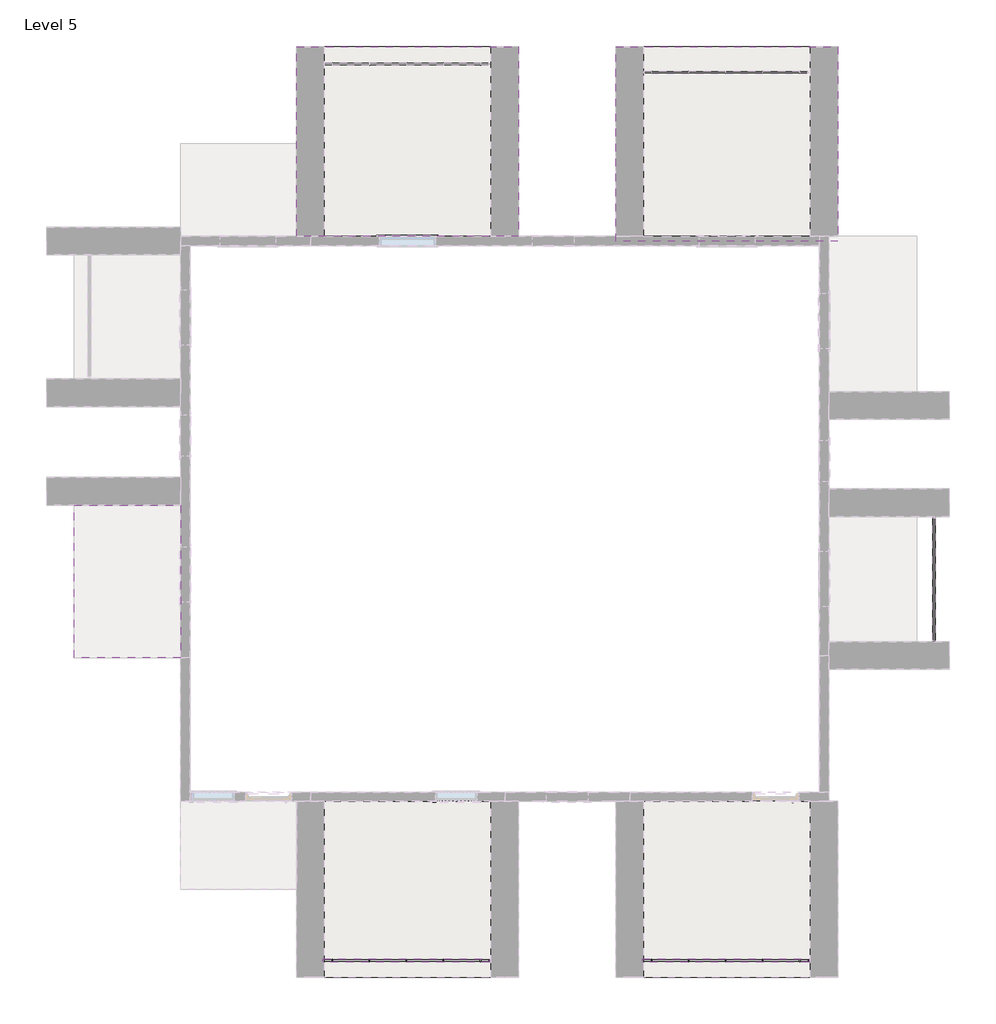
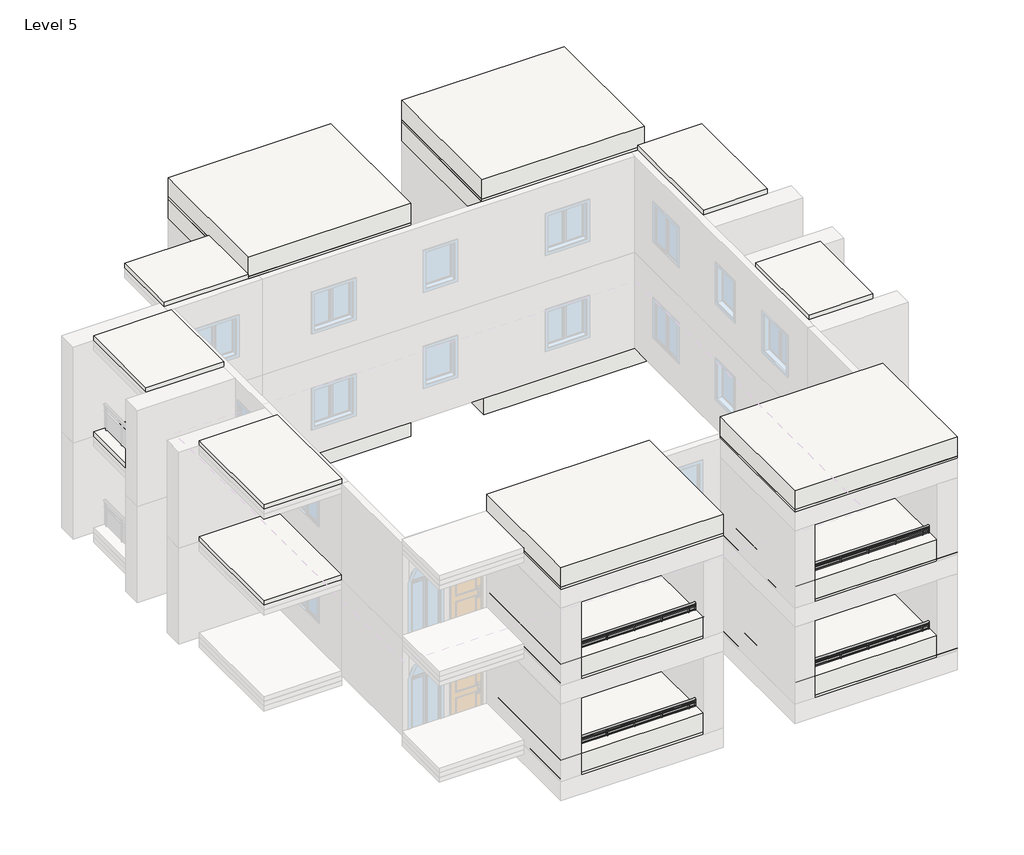
# One storey, part 3 of 4: 14 slabs, 5 railings.
"""IFC4 building model written with IfcOpenShell, lengths in millimetres."""

from ifc_helpers import new_model, si_unit, point, frame, origin, place, context, project, spatial, polyline, ellipse_curve, trimmed, outline, extrude, element, save
from ifc_brep_helpers import plane_surface, extruded_surface, advanced_brep

model = new_model("IFC4")

# Units and contexts
model_context = context("Model", 3, world=origin())
ifc_project = project(units=[si_unit("LENGTHUNIT", "METRE", prefix="MILLI")], contexts=[model_context])

# Site, building, storey
site = spatial("IfcSite", under=ifc_project)
building = spatial("IfcBuilding", under=site)
storey = spatial("IfcBuildingStorey", under=building, Name="Level 5", Elevation=12192.0)

# Railings
placement = place(None, origin())
element("IfcRailing", 1, ObjectType="Glass Panel - Bottom Fill", at=placement, inside=storey, context=model_context, shape_type="SolidModel", body=[
    advanced_brep(
    [(-9258.4937431, -9324.2034265, 13411.2), (-9258.4937431, -9400.4034265, 13411.2), (-5600.8937431, -9324.2034265, 13411.2), (-5600.8937431, -9400.4034265, 13411.2)],
    [
        (0, 1, ellipse_curve(frame((-9258.4937431, -9362.3034265, 13411.2), z_axis=(-1.0, 0.0, 0.0), x_axis=(0.0, -1.0, 0.0)), 38.1, 28.575)),
        (1, 0, ellipse_curve(frame((-9258.4937431, -9362.3034265, 13411.2), z_axis=(-1.0, 0.0, 0.0), x_axis=(0.0, -1.0, 0.0)), 38.1, 28.575)),
        (2, 3, ellipse_curve(frame((-5600.8937431, -9362.3034265, 13411.2), z_axis=(1.0, 0.0, 0.0), x_axis=(0.0, -1.0, 0.0)), 38.1, 28.575)),
        (3, 2, ellipse_curve(frame((-5600.8937431, -9362.3034265, 13411.2), z_axis=(1.0, 0.0, 0.0), x_axis=(0.0, -1.0, 0.0)), 38.1, 28.575)),
        (0, 2),
        (3, 1),
    ],
    [
        plane_surface(frame((-9258.4937431, -9362.3034265, 13411.2), z_axis=(-1.0, 0.0, 0.0), x_axis=(0.0, 1.0, 0.0))),
        plane_surface(frame((-5600.8937431, -9362.3034265, 13411.2), z_axis=(1.0, 0.0, 0.0), x_axis=(0.0, 1.0, 0.0))),
        extruded_surface(trimmed(ellipse_curve(frame((-5600.8937431, -9362.3034265, 13411.2), z_axis=(-1.0, 0.0, 0.0), x_axis=(0.0, -1.0, 0.0)), 38.1, 28.575), [point((-5600.8937431, -9324.2034265, 13411.2))], [point((-5600.8937431, -9400.4034265, 13411.2))], True, "CARTESIAN"), (-3657.5999999999995, 0.0, 0.0), 3657.5999999999995),
        extruded_surface(trimmed(ellipse_curve(frame((-5600.8937431, -9362.3034265, 13411.2), z_axis=(-1.0, 0.0, 0.0), x_axis=(0.0, -1.0, 0.0)), 38.1, 28.575), [point((-5600.8937431, -9400.4034265, 13411.2))], [point((-5600.8937431, -9324.2034265, 13411.2))], True, "CARTESIAN"), (-3657.5999999999995, 0.0, 0.0), 3657.5999999999995),
    ],
    [
        (0, [[1, 2]]),
        (1, [[3, 4]]),
        (2, [[-1, 5, -4, 6]]),
        (3, [[-2, -6, -3, -5]]),
    ],
),
    extrude(outline(polyline([(-9258.4937431, -9375.0034265), (-9258.4937431, -9349.6034265), (-5600.8937431, -9349.6034265), (-5600.8937431, -9375.0034265), (-9258.4937431, -9375.0034265)])), frame((0.0, 0.0, 13296.9), z_axis=(0.0, 0.0, 1.0), x_axis=(1.0, 0.0, 0.0)), (0.0, 0.0, 1.0), 25.4),
    extrude(outline(polyline([(-9258.4937431, -9375.0034265), (-9258.4937431, -9349.6034265), (-5600.8937431, -9349.6034265), (-5600.8937431, -9375.0034265), (-9258.4937431, -9375.0034265)])), frame((0.0, 0.0, 13195.3), z_axis=(0.0, 0.0, 1.0), x_axis=(1.0, 0.0, 0.0)), (0.0, 0.0, 1.0), 25.4),
    extrude(outline(polyline([(-5810.4437431, -9387.7034265), (-5810.4437431, -9336.9034265), (-5797.7437431, -9336.9034265), (-5797.7437431, -9387.7034265), (-5810.4437431, -9387.7034265)])), frame((0.0, 0.0, 12496.8), z_axis=(0.0, 0.0, 1.0), x_axis=(1.0, 0.0, 0.0)), (0.0, 0.0, 1.0), 885.6788223),
    extrude(outline(polyline([(-6616.8937431, -9355.7682695), (-5804.0937431, -9355.7682695), (-5804.0937431, -9362.1182695), (-6616.8937431, -9362.1182695), (-6616.8937431, -9355.7682695)])), frame((0.0, 0.0, 12598.4), z_axis=(0.0, 0.0, 1.0), x_axis=(1.0, 0.0, 0.0)), (0.0, 0.0, 1.0), 596.9),
    extrude(outline(polyline([(-6623.2437431, -9387.7034265), (-6623.2437431, -9336.9034265), (-6610.5437431, -9336.9034265), (-6610.5437431, -9387.7034265), (-6623.2437431, -9387.7034265)])), frame((0.0, 0.0, 12496.8), z_axis=(0.0, 0.0, 1.0), x_axis=(1.0, 0.0, 0.0)), (0.0, 0.0, 1.0), 885.6788223),
    extrude(outline(polyline([(-7429.6937431, -9355.7682695), (-6616.8937431, -9355.7682695), (-6616.8937431, -9362.1182695), (-7429.6937431, -9362.1182695), (-7429.6937431, -9355.7682695)])), frame((0.0, 0.0, 12598.4), z_axis=(0.0, 0.0, 1.0), x_axis=(1.0, 0.0, 0.0)), (0.0, 0.0, 1.0), 596.9),
    extrude(outline(polyline([(-7436.0437431, -9387.7034265), (-7436.0437431, -9336.9034265), (-7423.3437431, -9336.9034265), (-7423.3437431, -9387.7034265), (-7436.0437431, -9387.7034265)])), frame((0.0, 0.0, 12496.8), z_axis=(0.0, 0.0, 1.0), x_axis=(1.0, 0.0, 0.0)), (0.0, 0.0, 1.0), 885.6788223),
    extrude(outline(polyline([(-8242.4937431, -9355.7682695), (-7429.6937431, -9355.7682695), (-7429.6937431, -9362.1182695), (-8242.4937431, -9362.1182695), (-8242.4937431, -9355.7682695)])), frame((0.0, 0.0, 12598.4), z_axis=(0.0, 0.0, 1.0), x_axis=(1.0, 0.0, 0.0)), (0.0, 0.0, 1.0), 596.9),
    extrude(outline(polyline([(-8248.8437431, -9387.7034265), (-8248.8437431, -9336.9034265), (-8236.1437431, -9336.9034265), (-8236.1437431, -9387.7034265), (-8248.8437431, -9387.7034265)])), frame((0.0, 0.0, 12496.8), z_axis=(0.0, 0.0, 1.0), x_axis=(1.0, 0.0, 0.0)), (0.0, 0.0, 1.0), 885.6788223),
    extrude(outline(polyline([(-9055.2937431, -9355.7682695), (-8242.4937431, -9355.7682695), (-8242.4937431, -9362.1182695), (-9055.2937431, -9362.1182695), (-9055.2937431, -9355.7682695)])), frame((0.0, 0.0, 12598.4), z_axis=(0.0, 0.0, 1.0), x_axis=(1.0, 0.0, 0.0)), (0.0, 0.0, 1.0), 596.9),
    extrude(outline(polyline([(-9061.6437431, -9387.7034265), (-9061.6437431, -9336.9034265), (-9048.9437431, -9336.9034265), (-9048.9437431, -9387.7034265), (-9061.6437431, -9387.7034265)])), frame((0.0, 0.0, 12496.8), z_axis=(0.0, 0.0, 1.0), x_axis=(1.0, 0.0, 0.0)), (0.0, 0.0, 1.0), 885.6788223),
    extrude(outline(polyline([(-5613.5937431, -9371.8284265), (-5613.5937431, -9352.7784265), (-5594.5437431, -9352.7784265), (-5594.5437431, -9371.8284265), (-5613.5937431, -9371.8284265)])), frame((0.0, 0.0, 12496.8), z_axis=(0.0, 0.0, 1.0), x_axis=(1.0, 0.0, 0.0)), (0.0, 0.0, 1.0), 885.6788223),
    extrude(outline(polyline([(-9264.8437431, -9371.8284265), (-9264.8437431, -9352.7784265), (-9245.7937431, -9352.7784265), (-9245.7937431, -9371.8284265), (-9264.8437431, -9371.8284265)])), frame((0.0, 0.0, 12496.8), z_axis=(0.0, 0.0, 1.0), x_axis=(1.0, 0.0, 0.0)), (0.0, 0.0, 1.0), 885.6788223),
])
element("IfcRailing", 2, ObjectType="Glass Panel - Bottom Fill", at=placement, inside=storey, context=model_context, shape_type="SolidModel", body=[
    advanced_brep(
    [(-2248.0325613, -9324.2034265, 13406.1393423), (-2248.0325613, -9400.4034265, 13406.1393423), (1409.5674387, -9324.2034265, 13406.1393423), (1409.5674387, -9400.4034265, 13406.1393423)],
    [
        (0, 1, ellipse_curve(frame((-2248.0325613, -9362.3034265, 13406.1393423), z_axis=(-1.0, 0.0, 0.0), x_axis=(0.0, -1.0, 0.0)), 38.1, 28.575)),
        (1, 0, ellipse_curve(frame((-2248.0325613, -9362.3034265, 13406.1393423), z_axis=(-1.0, 0.0, 0.0), x_axis=(0.0, -1.0, 0.0)), 38.1, 28.575)),
        (2, 3, ellipse_curve(frame((1409.5674387, -9362.3034265, 13406.1393423), z_axis=(1.0, 0.0, 0.0), x_axis=(0.0, -1.0, 0.0)), 38.1, 28.575)),
        (3, 2, ellipse_curve(frame((1409.5674387, -9362.3034265, 13406.1393423), z_axis=(1.0, 0.0, 0.0), x_axis=(0.0, -1.0, 0.0)), 38.1, 28.575)),
        (0, 2),
        (3, 1),
    ],
    [
        plane_surface(frame((-2248.0325613, -9362.3034265, 13406.1393423), z_axis=(-1.0, 0.0, 0.0), x_axis=(0.0, 1.0, 0.0))),
        plane_surface(frame((1409.5674387, -9362.3034265, 13406.1393423), z_axis=(1.0, 0.0, 0.0), x_axis=(0.0, 1.0, 0.0))),
        extruded_surface(trimmed(ellipse_curve(frame((1409.5674387, -9362.3034265, 13406.1393423), z_axis=(-1.0, 0.0, 0.0), x_axis=(0.0, -1.0, 0.0)), 38.1, 28.575), [point((1409.5674387, -9324.2034265, 13406.1393423))], [point((1409.5674387, -9400.4034265, 13406.1393423))], True, "CARTESIAN"), (-3657.6, 0.0, 0.0), 3657.6),
        extruded_surface(trimmed(ellipse_curve(frame((1409.5674387, -9362.3034265, 13406.1393423), z_axis=(-1.0, 0.0, 0.0), x_axis=(0.0, -1.0, 0.0)), 38.1, 28.575), [point((1409.5674387, -9400.4034265, 13406.1393423))], [point((1409.5674387, -9324.2034265, 13406.1393423))], True, "CARTESIAN"), (-3657.6, 0.0, 0.0), 3657.6),
    ],
    [
        (0, [[1, 2]]),
        (1, [[3, 4]]),
        (2, [[-1, 5, -4, 6]]),
        (3, [[-2, -6, -3, -5]]),
    ],
),
    extrude(outline(polyline([(-2248.0325613, -9375.0034265), (-2248.0325613, -9349.6034265), (1409.5674387, -9349.6034265), (1409.5674387, -9375.0034265), (-2248.0325613, -9375.0034265)])), frame((0.0, 0.0, 13291.8393423), z_axis=(0.0, 0.0, 1.0), x_axis=(1.0, 0.0, 0.0)), (0.0, 0.0, 1.0), 25.4),
    extrude(outline(polyline([(-2248.0325613, -9375.0034265), (-2248.0325613, -9349.6034265), (1409.5674387, -9349.6034265), (1409.5674387, -9375.0034265), (-2248.0325613, -9375.0034265)])), frame((0.0, 0.0, 13190.2393423), z_axis=(0.0, 0.0, 1.0), x_axis=(1.0, 0.0, 0.0)), (0.0, 0.0, 1.0), 25.4),
    extrude(outline(polyline([(1200.0174387, -9387.7034265), (1200.0174387, -9336.9034265), (1212.7174387, -9336.9034265), (1212.7174387, -9387.7034265), (1200.0174387, -9387.7034265)])), frame((0.0, 0.0, 12491.7393423), z_axis=(0.0, 0.0, 1.0), x_axis=(1.0, 0.0, 0.0)), (0.0, 0.0, 1.0), 885.6788223),
    extrude(outline(polyline([(393.5674387, -9355.7682695), (1206.3674387, -9355.7682695), (1206.3674387, -9362.1182695), (393.5674387, -9362.1182695), (393.5674387, -9355.7682695)])), frame((0.0, 0.0, 12593.3393423), z_axis=(0.0, 0.0, 1.0), x_axis=(1.0, 0.0, 0.0)), (0.0, 0.0, 1.0), 596.9),
    extrude(outline(polyline([(387.2174387, -9387.7034265), (387.2174387, -9336.9034265), (399.9174387, -9336.9034265), (399.9174387, -9387.7034265), (387.2174387, -9387.7034265)])), frame((0.0, 0.0, 12491.7393423), z_axis=(0.0, 0.0, 1.0), x_axis=(1.0, 0.0, 0.0)), (0.0, 0.0, 1.0), 885.6788223),
    extrude(outline(polyline([(-419.2325613, -9355.7682695), (393.5674387, -9355.7682695), (393.5674387, -9362.1182695), (-419.2325613, -9362.1182695), (-419.2325613, -9355.7682695)])), frame((0.0, 0.0, 12593.3393423), z_axis=(0.0, 0.0, 1.0), x_axis=(1.0, 0.0, 0.0)), (0.0, 0.0, 1.0), 596.9),
    extrude(outline(polyline([(-425.5825613, -9387.7034265), (-425.5825613, -9336.9034265), (-412.8825613, -9336.9034265), (-412.8825613, -9387.7034265), (-425.5825613, -9387.7034265)])), frame((0.0, 0.0, 12491.7393423), z_axis=(0.0, 0.0, 1.0), x_axis=(1.0, 0.0, 0.0)), (0.0, 0.0, 1.0), 885.6788223),
    extrude(outline(polyline([(-1232.0325613, -9355.7682695), (-419.2325613, -9355.7682695), (-419.2325613, -9362.1182695), (-1232.0325613, -9362.1182695), (-1232.0325613, -9355.7682695)])), frame((0.0, 0.0, 12593.3393423), z_axis=(0.0, 0.0, 1.0), x_axis=(1.0, 0.0, 0.0)), (0.0, 0.0, 1.0), 596.9),
    extrude(outline(polyline([(-1238.3825613, -9387.7034265), (-1238.3825613, -9336.9034265), (-1225.6825613, -9336.9034265), (-1225.6825613, -9387.7034265), (-1238.3825613, -9387.7034265)])), frame((0.0, 0.0, 12491.7393423), z_axis=(0.0, 0.0, 1.0), x_axis=(1.0, 0.0, 0.0)), (0.0, 0.0, 1.0), 885.6788223),
    extrude(outline(polyline([(-2044.8325613, -9355.7682695), (-1232.0325613, -9355.7682695), (-1232.0325613, -9362.1182695), (-2044.8325613, -9362.1182695), (-2044.8325613, -9355.7682695)])), frame((0.0, 0.0, 12593.3393423), z_axis=(0.0, 0.0, 1.0), x_axis=(1.0, 0.0, 0.0)), (0.0, 0.0, 1.0), 596.9),
    extrude(outline(polyline([(-2051.1825613, -9387.7034265), (-2051.1825613, -9336.9034265), (-2038.4825613, -9336.9034265), (-2038.4825613, -9387.7034265), (-2051.1825613, -9387.7034265)])), frame((0.0, 0.0, 12491.7393423), z_axis=(0.0, 0.0, 1.0), x_axis=(1.0, 0.0, 0.0)), (0.0, 0.0, 1.0), 885.6788223),
    extrude(outline(polyline([(1396.8674387, -9371.8284265), (1396.8674387, -9352.7784265), (1415.9174387, -9352.7784265), (1415.9174387, -9371.8284265), (1396.8674387, -9371.8284265)])), frame((0.0, 0.0, 12491.7393423), z_axis=(0.0, 0.0, 1.0), x_axis=(1.0, 0.0, 0.0)), (0.0, 0.0, 1.0), 885.6788223),
    extrude(outline(polyline([(-2254.3825613, -9371.8284265), (-2254.3825613, -9352.7784265), (-2235.3325613, -9352.7784265), (-2235.3325613, -9371.8284265), (-2254.3825613, -9371.8284265)])), frame((0.0, 0.0, 12491.7393423), z_axis=(0.0, 0.0, 1.0), x_axis=(1.0, 0.0, 0.0)), (0.0, 0.0, 1.0), 885.6788223),
])
element("IfcRailing", 3, ObjectType="Glass Panel - Bottom Fill", at=placement, inside=storey, context=model_context, shape_type="SolidModel", body=[
    advanced_brep(
    [(4190.8062569, 350.013611, 13411.2), (4114.6062569, 350.013611, 13411.2), (4190.8062569, -2342.386389, 13411.2), (4114.6062569, -2342.386389, 13411.2)],
    [
        (0, 1, ellipse_curve(frame((4152.7062569, 350.013611, 13411.2), z_axis=(0.0, 1.0, 0.0), x_axis=(-1.0, 0.0, 0.0)), 38.1, 28.575)),
        (1, 0, ellipse_curve(frame((4152.7062569, 350.013611, 13411.2), z_axis=(0.0, 1.0, 0.0), x_axis=(-1.0, 0.0, 0.0)), 38.1, 28.575)),
        (2, 3, ellipse_curve(frame((4152.7062569, -2342.386389, 13411.2), z_axis=(0.0, -1.0, 0.0), x_axis=(-1.0, 0.0, 0.0)), 38.1, 28.575)),
        (3, 2, ellipse_curve(frame((4152.7062569, -2342.386389, 13411.2), z_axis=(0.0, -1.0, 0.0), x_axis=(-1.0, 0.0, 0.0)), 38.1, 28.575)),
        (0, 2),
        (3, 1),
    ],
    [
        plane_surface(frame((4152.7062569, 350.013611, 13411.2), z_axis=(0.0, 1.0, 0.0), x_axis=(0.0, 0.0, -1.0))),
        plane_surface(frame((4152.7062569, -2342.386389, 13411.2), z_axis=(0.0, -1.0, 0.0), x_axis=(0.0, 0.0, -1.0))),
        extruded_surface(trimmed(ellipse_curve(frame((4152.7062569, -2342.386389, 13411.2), z_axis=(0.0, 1.0, 0.0), x_axis=(-1.0, 0.0, 0.0)), 38.1, 28.575), [point((4190.8062569, -2342.386389, 13411.2))], [point((4114.6062569, -2342.386389, 13411.2))], True, "CARTESIAN"), (0.0, 2692.3999999999996, 0.0), 2692.3999999999996),
        extruded_surface(trimmed(ellipse_curve(frame((4152.7062569, -2342.386389, 13411.2), z_axis=(0.0, 1.0, 0.0), x_axis=(-1.0, 0.0, 0.0)), 38.1, 28.575), [point((4114.6062569, -2342.386389, 13411.2))], [point((4190.8062569, -2342.386389, 13411.2))], True, "CARTESIAN"), (0.0, 2692.3999999999996, 0.0), 2692.3999999999996),
    ],
    [
        (0, [[1, 2]]),
        (1, [[3, 4]]),
        (2, [[-1, 5, -4, 6]]),
        (3, [[-2, -6, -3, -5]]),
    ],
),
    extrude(outline(polyline([(4140.0062569, 350.013611), (4165.4062569, 350.013611), (4165.4062569, -2342.386389), (4140.0062569, -2342.386389), (4140.0062569, 350.013611)])), frame((0.0, 0.0, 13296.9), z_axis=(0.0, 0.0, 1.0), x_axis=(1.0, 0.0, 0.0)), (0.0, 0.0, 1.0), 25.4),
    extrude(outline(polyline([(4140.0062569, 350.013611), (4165.4062569, 350.013611), (4165.4062569, -2342.386389), (4140.0062569, -2342.386389), (4140.0062569, 350.013611)])), frame((0.0, 0.0, 13195.3), z_axis=(0.0, 0.0, 1.0), x_axis=(1.0, 0.0, 0.0)), (0.0, 0.0, 1.0), 25.4),
    extrude(outline(polyline([(4127.3062569, -2209.036389), (4178.1062569, -2209.036389), (4178.1062569, -2221.736389), (4127.3062569, -2221.736389), (4127.3062569, -2209.036389)])), frame((0.0, 0.0, 12496.8), z_axis=(0.0, 0.0, 1.0), x_axis=(1.0, 0.0, 0.0)), (0.0, 0.0, 1.0), 885.6788223),
    extrude(outline(polyline([(4159.2414139, -1402.586389), (4159.2414139, -2215.386389), (4152.8914139, -2215.386389), (4152.8914139, -1402.586389), (4159.2414139, -1402.586389)])), frame((0.0, 0.0, 12598.4), z_axis=(0.0, 0.0, 1.0), x_axis=(1.0, 0.0, 0.0)), (0.0, 0.0, 1.0), 596.9),
    extrude(outline(polyline([(4127.3062569, -1396.236389), (4178.1062569, -1396.236389), (4178.1062569, -1408.936389), (4127.3062569, -1408.936389), (4127.3062569, -1396.236389)])), frame((0.0, 0.0, 12496.8), z_axis=(0.0, 0.0, 1.0), x_axis=(1.0, 0.0, 0.0)), (0.0, 0.0, 1.0), 885.6788223),
    extrude(outline(polyline([(4159.2414139, -589.786389), (4159.2414139, -1402.586389), (4152.8914139, -1402.586389), (4152.8914139, -589.786389), (4159.2414139, -589.786389)])), frame((0.0, 0.0, 12598.4), z_axis=(0.0, 0.0, 1.0), x_axis=(1.0, 0.0, 0.0)), (0.0, 0.0, 1.0), 596.9),
    extrude(outline(polyline([(4127.3062569, -583.436389), (4178.1062569, -583.436389), (4178.1062569, -596.136389), (4127.3062569, -596.136389), (4127.3062569, -583.436389)])), frame((0.0, 0.0, 12496.8), z_axis=(0.0, 0.0, 1.0), x_axis=(1.0, 0.0, 0.0)), (0.0, 0.0, 1.0), 885.6788223),
    extrude(outline(polyline([(4159.2414139, 223.013611), (4159.2414139, -589.786389), (4152.8914139, -589.786389), (4152.8914139, 223.013611), (4159.2414139, 223.013611)])), frame((0.0, 0.0, 12598.4), z_axis=(0.0, 0.0, 1.0), x_axis=(1.0, 0.0, 0.0)), (0.0, 0.0, 1.0), 596.9),
    extrude(outline(polyline([(4127.3062569, 229.363611), (4178.1062569, 229.363611), (4178.1062569, 216.663611), (4127.3062569, 216.663611), (4127.3062569, 229.363611)])), frame((0.0, 0.0, 12496.8), z_axis=(0.0, 0.0, 1.0), x_axis=(1.0, 0.0, 0.0)), (0.0, 0.0, 1.0), 885.6788223),
    extrude(outline(polyline([(4143.1812569, -2329.686389), (4162.2312569, -2329.686389), (4162.2312569, -2348.736389), (4143.1812569, -2348.736389), (4143.1812569, -2329.686389)])), frame((0.0, 0.0, 12496.8), z_axis=(0.0, 0.0, 1.0), x_axis=(1.0, 0.0, 0.0)), (0.0, 0.0, 1.0), 885.6788223),
    extrude(outline(polyline([(4143.1812569, 356.363611), (4162.2312569, 356.363611), (4162.2312569, 337.313611), (4143.1812569, 337.313611), (4143.1812569, 356.363611)])), frame((0.0, 0.0, 12496.8), z_axis=(0.0, 0.0, 1.0), x_axis=(1.0, 0.0, 0.0)), (0.0, 0.0, 1.0), 885.6788223),
])
element("IfcRailing", 4, ObjectType="Glass Panel - Bottom Fill", at=placement, inside=storey, context=model_context, shape_type="SolidModel", body=[
    advanced_brep(
    [(-9258.4937431, -9324.2034265, 16459.2), (-9258.4937431, -9400.4034265, 16459.2), (-5600.8937431, -9324.2034265, 16459.2), (-5600.8937431, -9400.4034265, 16459.2)],
    [
        (0, 1, ellipse_curve(frame((-9258.4937431, -9362.3034265, 16459.2), z_axis=(-1.0, 0.0, 0.0), x_axis=(0.0, -1.0, 0.0)), 38.1, 28.575)),
        (1, 0, ellipse_curve(frame((-9258.4937431, -9362.3034265, 16459.2), z_axis=(-1.0, 0.0, 0.0), x_axis=(0.0, -1.0, 0.0)), 38.1, 28.575)),
        (2, 3, ellipse_curve(frame((-5600.8937431, -9362.3034265, 16459.2), z_axis=(1.0, 0.0, 0.0), x_axis=(0.0, -1.0, 0.0)), 38.1, 28.575)),
        (3, 2, ellipse_curve(frame((-5600.8937431, -9362.3034265, 16459.2), z_axis=(1.0, 0.0, 0.0), x_axis=(0.0, -1.0, 0.0)), 38.1, 28.575)),
        (0, 2),
        (3, 1),
    ],
    [
        plane_surface(frame((-9258.4937431, -9362.3034265, 16459.2), z_axis=(-1.0, 0.0, 0.0), x_axis=(0.0, 1.0, 0.0))),
        plane_surface(frame((-5600.8937431, -9362.3034265, 16459.2), z_axis=(1.0, 0.0, 0.0), x_axis=(0.0, 1.0, 0.0))),
        extruded_surface(trimmed(ellipse_curve(frame((-5600.8937431, -9362.3034265, 16459.2), z_axis=(-1.0, 0.0, 0.0), x_axis=(0.0, -1.0, 0.0)), 38.1, 28.575), [point((-5600.8937431, -9324.2034265, 16459.2))], [point((-5600.8937431, -9400.4034265, 16459.2))], True, "CARTESIAN"), (-3657.5999999999995, 0.0, 0.0), 3657.5999999999995),
        extruded_surface(trimmed(ellipse_curve(frame((-5600.8937431, -9362.3034265, 16459.2), z_axis=(-1.0, 0.0, 0.0), x_axis=(0.0, -1.0, 0.0)), 38.1, 28.575), [point((-5600.8937431, -9400.4034265, 16459.2))], [point((-5600.8937431, -9324.2034265, 16459.2))], True, "CARTESIAN"), (-3657.5999999999995, 0.0, 0.0), 3657.5999999999995),
    ],
    [
        (0, [[1, 2]]),
        (1, [[3, 4]]),
        (2, [[-1, 5, -4, 6]]),
        (3, [[-2, -6, -3, -5]]),
    ],
),
    extrude(outline(polyline([(-9258.4937431, -9375.0034265), (-9258.4937431, -9349.6034265), (-5600.8937431, -9349.6034265), (-5600.8937431, -9375.0034265), (-9258.4937431, -9375.0034265)])), frame((0.0, 0.0, 16344.9), z_axis=(0.0, 0.0, 1.0), x_axis=(1.0, 0.0, 0.0)), (0.0, 0.0, 1.0), 25.4),
    extrude(outline(polyline([(-9258.4937431, -9375.0034265), (-9258.4937431, -9349.6034265), (-5600.8937431, -9349.6034265), (-5600.8937431, -9375.0034265), (-9258.4937431, -9375.0034265)])), frame((0.0, 0.0, 16243.3), z_axis=(0.0, 0.0, 1.0), x_axis=(1.0, 0.0, 0.0)), (0.0, 0.0, 1.0), 25.4),
    extrude(outline(polyline([(-5810.4437431, -9387.7034265), (-5810.4437431, -9336.9034265), (-5797.7437431, -9336.9034265), (-5797.7437431, -9387.7034265), (-5810.4437431, -9387.7034265)])), frame((0.0, 0.0, 15544.8), z_axis=(0.0, 0.0, 1.0), x_axis=(1.0, 0.0, 0.0)), (0.0, 0.0, 1.0), 885.6788223),
    extrude(outline(polyline([(-6616.8937431, -9355.7682695), (-5804.0937431, -9355.7682695), (-5804.0937431, -9362.1182695), (-6616.8937431, -9362.1182695), (-6616.8937431, -9355.7682695)])), frame((0.0, 0.0, 15646.4), z_axis=(0.0, 0.0, 1.0), x_axis=(1.0, 0.0, 0.0)), (0.0, 0.0, 1.0), 596.9),
    extrude(outline(polyline([(-6623.2437431, -9387.7034265), (-6623.2437431, -9336.9034265), (-6610.5437431, -9336.9034265), (-6610.5437431, -9387.7034265), (-6623.2437431, -9387.7034265)])), frame((0.0, 0.0, 15544.8), z_axis=(0.0, 0.0, 1.0), x_axis=(1.0, 0.0, 0.0)), (0.0, 0.0, 1.0), 885.6788223),
    extrude(outline(polyline([(-7429.6937431, -9355.7682695), (-6616.8937431, -9355.7682695), (-6616.8937431, -9362.1182695), (-7429.6937431, -9362.1182695), (-7429.6937431, -9355.7682695)])), frame((0.0, 0.0, 15646.4), z_axis=(0.0, 0.0, 1.0), x_axis=(1.0, 0.0, 0.0)), (0.0, 0.0, 1.0), 596.9),
    extrude(outline(polyline([(-7436.0437431, -9387.7034265), (-7436.0437431, -9336.9034265), (-7423.3437431, -9336.9034265), (-7423.3437431, -9387.7034265), (-7436.0437431, -9387.7034265)])), frame((0.0, 0.0, 15544.8), z_axis=(0.0, 0.0, 1.0), x_axis=(1.0, 0.0, 0.0)), (0.0, 0.0, 1.0), 885.6788223),
    extrude(outline(polyline([(-8242.4937431, -9355.7682695), (-7429.6937431, -9355.7682695), (-7429.6937431, -9362.1182695), (-8242.4937431, -9362.1182695), (-8242.4937431, -9355.7682695)])), frame((0.0, 0.0, 15646.4), z_axis=(0.0, 0.0, 1.0), x_axis=(1.0, 0.0, 0.0)), (0.0, 0.0, 1.0), 596.9),
    extrude(outline(polyline([(-8248.8437431, -9387.7034265), (-8248.8437431, -9336.9034265), (-8236.1437431, -9336.9034265), (-8236.1437431, -9387.7034265), (-8248.8437431, -9387.7034265)])), frame((0.0, 0.0, 15544.8), z_axis=(0.0, 0.0, 1.0), x_axis=(1.0, 0.0, 0.0)), (0.0, 0.0, 1.0), 885.6788223),
    extrude(outline(polyline([(-9055.2937431, -9355.7682695), (-8242.4937431, -9355.7682695), (-8242.4937431, -9362.1182695), (-9055.2937431, -9362.1182695), (-9055.2937431, -9355.7682695)])), frame((0.0, 0.0, 15646.4), z_axis=(0.0, 0.0, 1.0), x_axis=(1.0, 0.0, 0.0)), (0.0, 0.0, 1.0), 596.9),
    extrude(outline(polyline([(-9061.6437431, -9387.7034265), (-9061.6437431, -9336.9034265), (-9048.9437431, -9336.9034265), (-9048.9437431, -9387.7034265), (-9061.6437431, -9387.7034265)])), frame((0.0, 0.0, 15544.8), z_axis=(0.0, 0.0, 1.0), x_axis=(1.0, 0.0, 0.0)), (0.0, 0.0, 1.0), 885.6788223),
    extrude(outline(polyline([(-5613.5937431, -9371.8284265), (-5613.5937431, -9352.7784265), (-5594.5437431, -9352.7784265), (-5594.5437431, -9371.8284265), (-5613.5937431, -9371.8284265)])), frame((0.0, 0.0, 15544.8), z_axis=(0.0, 0.0, 1.0), x_axis=(1.0, 0.0, 0.0)), (0.0, 0.0, 1.0), 885.6788223),
    extrude(outline(polyline([(-9264.8437431, -9371.8284265), (-9264.8437431, -9352.7784265), (-9245.7937431, -9352.7784265), (-9245.7937431, -9371.8284265), (-9264.8437431, -9371.8284265)])), frame((0.0, 0.0, 15544.8), z_axis=(0.0, 0.0, 1.0), x_axis=(1.0, 0.0, 0.0)), (0.0, 0.0, 1.0), 885.6788223),
])
element("IfcRailing", 5, ObjectType="Glass Panel - Bottom Fill", at=placement, inside=storey, context=model_context, shape_type="SolidModel", body=[
    advanced_brep(
    [(-2248.0325613, -9324.2034265, 16454.1393423), (-2248.0325613, -9400.4034265, 16454.1393423), (1409.5674387, -9324.2034265, 16454.1393423), (1409.5674387, -9400.4034265, 16454.1393423)],
    [
        (0, 1, ellipse_curve(frame((-2248.0325613, -9362.3034265, 16454.1393423), z_axis=(-1.0, 0.0, 0.0), x_axis=(0.0, -1.0, 0.0)), 38.1, 28.575)),
        (1, 0, ellipse_curve(frame((-2248.0325613, -9362.3034265, 16454.1393423), z_axis=(-1.0, 0.0, 0.0), x_axis=(0.0, -1.0, 0.0)), 38.1, 28.575)),
        (2, 3, ellipse_curve(frame((1409.5674387, -9362.3034265, 16454.1393423), z_axis=(1.0, 0.0, 0.0), x_axis=(0.0, -1.0, 0.0)), 38.1, 28.575)),
        (3, 2, ellipse_curve(frame((1409.5674387, -9362.3034265, 16454.1393423), z_axis=(1.0, 0.0, 0.0), x_axis=(0.0, -1.0, 0.0)), 38.1, 28.575)),
        (0, 2),
        (3, 1),
    ],
    [
        plane_surface(frame((-2248.0325613, -9362.3034265, 16454.1393423), z_axis=(-1.0, 0.0, 0.0), x_axis=(0.0, 1.0, 0.0))),
        plane_surface(frame((1409.5674387, -9362.3034265, 16454.1393423), z_axis=(1.0, 0.0, 0.0), x_axis=(0.0, 1.0, 0.0))),
        extruded_surface(trimmed(ellipse_curve(frame((1409.5674387, -9362.3034265, 16454.1393423), z_axis=(-1.0, 0.0, 0.0), x_axis=(0.0, -1.0, 0.0)), 38.1, 28.575), [point((1409.5674387, -9324.2034265, 16454.1393423))], [point((1409.5674387, -9400.4034265, 16454.1393423))], True, "CARTESIAN"), (-3657.6, 0.0, 0.0), 3657.6),
        extruded_surface(trimmed(ellipse_curve(frame((1409.5674387, -9362.3034265, 16454.1393423), z_axis=(-1.0, 0.0, 0.0), x_axis=(0.0, -1.0, 0.0)), 38.1, 28.575), [point((1409.5674387, -9400.4034265, 16454.1393423))], [point((1409.5674387, -9324.2034265, 16454.1393423))], True, "CARTESIAN"), (-3657.6, 0.0, 0.0), 3657.6),
    ],
    [
        (0, [[1, 2]]),
        (1, [[3, 4]]),
        (2, [[-1, 5, -4, 6]]),
        (3, [[-2, -6, -3, -5]]),
    ],
),
    extrude(outline(polyline([(-2248.0325613, -9375.0034265), (-2248.0325613, -9349.6034265), (1409.5674387, -9349.6034265), (1409.5674387, -9375.0034265), (-2248.0325613, -9375.0034265)])), frame((0.0, 0.0, 16339.8393423), z_axis=(0.0, 0.0, 1.0), x_axis=(1.0, 0.0, 0.0)), (0.0, 0.0, 1.0), 25.4),
    extrude(outline(polyline([(-2248.0325613, -9375.0034265), (-2248.0325613, -9349.6034265), (1409.5674387, -9349.6034265), (1409.5674387, -9375.0034265), (-2248.0325613, -9375.0034265)])), frame((0.0, 0.0, 16238.2393423), z_axis=(0.0, 0.0, 1.0), x_axis=(1.0, 0.0, 0.0)), (0.0, 0.0, 1.0), 25.4),
    extrude(outline(polyline([(1200.0174387, -9387.7034265), (1200.0174387, -9336.9034265), (1212.7174387, -9336.9034265), (1212.7174387, -9387.7034265), (1200.0174387, -9387.7034265)])), frame((0.0, 0.0, 15539.7393423), z_axis=(0.0, 0.0, 1.0), x_axis=(1.0, 0.0, 0.0)), (0.0, 0.0, 1.0), 885.6788223),
    extrude(outline(polyline([(393.5674387, -9355.7682695), (1206.3674387, -9355.7682695), (1206.3674387, -9362.1182695), (393.5674387, -9362.1182695), (393.5674387, -9355.7682695)])), frame((0.0, 0.0, 15641.3393423), z_axis=(0.0, 0.0, 1.0), x_axis=(1.0, 0.0, 0.0)), (0.0, 0.0, 1.0), 596.9),
    extrude(outline(polyline([(387.2174387, -9387.7034265), (387.2174387, -9336.9034265), (399.9174387, -9336.9034265), (399.9174387, -9387.7034265), (387.2174387, -9387.7034265)])), frame((0.0, 0.0, 15539.7393423), z_axis=(0.0, 0.0, 1.0), x_axis=(1.0, 0.0, 0.0)), (0.0, 0.0, 1.0), 885.6788223),
    extrude(outline(polyline([(-419.2325613, -9355.7682695), (393.5674387, -9355.7682695), (393.5674387, -9362.1182695), (-419.2325613, -9362.1182695), (-419.2325613, -9355.7682695)])), frame((0.0, 0.0, 15641.3393423), z_axis=(0.0, 0.0, 1.0), x_axis=(1.0, 0.0, 0.0)), (0.0, 0.0, 1.0), 596.9),
    extrude(outline(polyline([(-425.5825613, -9387.7034265), (-425.5825613, -9336.9034265), (-412.8825613, -9336.9034265), (-412.8825613, -9387.7034265), (-425.5825613, -9387.7034265)])), frame((0.0, 0.0, 15539.7393423), z_axis=(0.0, 0.0, 1.0), x_axis=(1.0, 0.0, 0.0)), (0.0, 0.0, 1.0), 885.6788223),
    extrude(outline(polyline([(-1232.0325613, -9355.7682695), (-419.2325613, -9355.7682695), (-419.2325613, -9362.1182695), (-1232.0325613, -9362.1182695), (-1232.0325613, -9355.7682695)])), frame((0.0, 0.0, 15641.3393423), z_axis=(0.0, 0.0, 1.0), x_axis=(1.0, 0.0, 0.0)), (0.0, 0.0, 1.0), 596.9),
    extrude(outline(polyline([(-1238.3825613, -9387.7034265), (-1238.3825613, -9336.9034265), (-1225.6825613, -9336.9034265), (-1225.6825613, -9387.7034265), (-1238.3825613, -9387.7034265)])), frame((0.0, 0.0, 15539.7393423), z_axis=(0.0, 0.0, 1.0), x_axis=(1.0, 0.0, 0.0)), (0.0, 0.0, 1.0), 885.6788223),
    extrude(outline(polyline([(-2044.8325613, -9355.7682695), (-1232.0325613, -9355.7682695), (-1232.0325613, -9362.1182695), (-2044.8325613, -9362.1182695), (-2044.8325613, -9355.7682695)])), frame((0.0, 0.0, 15641.3393423), z_axis=(0.0, 0.0, 1.0), x_axis=(1.0, 0.0, 0.0)), (0.0, 0.0, 1.0), 596.9),
    extrude(outline(polyline([(-2051.1825613, -9387.7034265), (-2051.1825613, -9336.9034265), (-2038.4825613, -9336.9034265), (-2038.4825613, -9387.7034265), (-2051.1825613, -9387.7034265)])), frame((0.0, 0.0, 15539.7393423), z_axis=(0.0, 0.0, 1.0), x_axis=(1.0, 0.0, 0.0)), (0.0, 0.0, 1.0), 885.6788223),
    extrude(outline(polyline([(1396.8674387, -9371.8284265), (1396.8674387, -9352.7784265), (1415.9174387, -9352.7784265), (1415.9174387, -9371.8284265), (1396.8674387, -9371.8284265)])), frame((0.0, 0.0, 15539.7393423), z_axis=(0.0, 0.0, 1.0), x_axis=(1.0, 0.0, 0.0)), (0.0, 0.0, 1.0), 885.6788223),
    extrude(outline(polyline([(-2254.3825613, -9371.8284265), (-2254.3825613, -9352.7784265), (-2235.3325613, -9352.7784265), (-2235.3325613, -9371.8284265), (-2254.3825613, -9371.8284265)])), frame((0.0, 0.0, 15539.7393423), z_axis=(0.0, 0.0, 1.0), x_axis=(1.0, 0.0, 0.0)), (0.0, 0.0, 1.0), 885.6788223),
])

# Slabs
element("IfcSlab", 6, ObjectType="Generic - 2'", at=placement, inside=storey, context=model_context, shape_type="SweptSolid", body=[
    extrude(outline(polyline([(-4965.8937431, 10687.813611), (-4965.8937431, 6522.213611), (-9842.6937431, 6522.213611), (-9842.6937431, 10687.813611), (-4965.8937431, 10687.813611)])), frame((0.0, 0.0, 11887.2), z_axis=(0.0, 0.0, 1.0), x_axis=(1.0, 0.0, 0.0)), (0.0, 0.0, 1.0), 609.6),
])
element("IfcSlab", 7, ObjectType="Generic - 2'", at=placement, inside=storey, context=model_context, shape_type="SweptSolid", body=[
    extrude(outline(polyline([(-4965.8937431, 10687.813611), (-4965.8937431, 6522.213611), (-9842.6937431, 6522.213611), (-9842.6937431, 10687.813611), (-4965.8937431, 10687.813611)])), frame((0.0, 0.0, 14935.2), z_axis=(0.0, 0.0, 1.0), x_axis=(1.0, 0.0, 0.0)), (0.0, 0.0, 1.0), 609.6),
])
element("IfcSlab", 8, ObjectType="Generic - 2'", at=placement, inside=storey, context=model_context, shape_type="SweptSolid", body=[
    extrude(outline(polyline([(-4965.8937431, 10687.813611), (-4965.8937431, 6522.213611), (-9842.6937431, 6522.213611), (-9842.6937431, 10687.813611), (-4965.8937431, 10687.813611)])), frame((0.0, 0.0, 17983.2), z_axis=(0.0, 0.0, 1.0), x_axis=(1.0, 0.0, 0.0)), (0.0, 0.0, 1.0), 609.6),
])
element("IfcSlab", 9, ObjectType="Generic - 2' 2", at=placement, inside=storey, context=model_context, shape_type="SweptSolid", body=[
    extrude(outline(polyline([(2044.5062569, 10687.813611), (2044.5062569, 6420.613611), (-2832.2937431, 6420.613611), (-2832.2937431, 10687.813611), (2044.5062569, 10687.813611)])), frame((0.0, 0.0, 11887.2), z_axis=(0.0, 0.0, 1.0), x_axis=(1.0, 0.0, 0.0)), (0.0, 0.0, 1.0), 609.6),
])
element("IfcSlab", 10, ObjectType="Generic - 2' 2", at=placement, inside=storey, context=model_context, shape_type="SweptSolid", body=[
    extrude(outline(polyline([(2044.5062569, 10687.813611), (2044.5062569, 6420.613611), (-2832.2937431, 6420.613611), (-2832.2937431, 10687.813611), (2044.5062569, 10687.813611)])), frame((0.0, 0.0, 14935.2), z_axis=(0.0, 0.0, 1.0), x_axis=(1.0, 0.0, 0.0)), (0.0, 0.0, 1.0), 609.6),
])
element("IfcSlab", 11, ObjectType="Generic - 2' 2", at=placement, inside=storey, context=model_context, shape_type="SweptSolid", body=[
    extrude(outline(polyline([(2044.5062569, 10687.813611), (2044.5062569, 6420.613611), (-2832.2937431, 6420.613611), (-2832.2937431, 10687.813611), (2044.5062569, 10687.813611)])), frame((0.0, 0.0, 17983.2), z_axis=(0.0, 0.0, 1.0), x_axis=(1.0, 0.0, 0.0)), (0.0, 0.0, 1.0), 609.6),
])
element("IfcSlab", 12, ObjectType="Generic - 2' 3", at=placement, inside=storey, context=model_context, shape_type="SweptSolid", body=[
    extrude(outline(polyline([(-4965.8937431, 6522.213611), (-9842.6937431, 6522.213611), (-9842.6937431, 10687.813611), (-4965.8937431, 10687.813611), (-4965.8937431, 6522.213611)])), frame((0.0, 0.0, 12496.8), z_axis=(0.0, 0.0, 1.0), x_axis=(1.0, 0.0, 0.0)), (0.0, 0.0, 1.0), 76.2),
    extrude(outline(polyline([(2044.5062569, 6522.213611), (-2832.2937431, 6522.213611), (-2832.2937431, 10687.813611), (2044.5062569, 10687.813611), (2044.5062569, 6522.213611)])), frame((0.0, 0.0, 12496.8), z_axis=(0.0, 0.0, 1.0), x_axis=(1.0, 0.0, 0.0)), (0.0, 0.0, 1.0), 76.2),
    extrude(outline(polyline([(-4965.8937431, -5872.986389), (-4965.8937431, -9733.786389), (-9842.6937431, -9733.786389), (-9842.6937431, -5872.986389), (-4965.8937431, -5872.986389)])), frame((0.0, 0.0, 12496.8), z_axis=(0.0, 0.0, 1.0), x_axis=(1.0, 0.0, 0.0)), (0.0, 0.0, 1.0), 76.2),
    extrude(outline(polyline([(2044.5062569, -5872.986389), (2044.5062569, -9733.786389), (-2832.2937431, -9733.786389), (-2832.2937431, -5872.986389), (2044.5062569, -5872.986389)])), frame((0.0, 0.0, 12496.8), z_axis=(0.0, 0.0, 1.0), x_axis=(1.0, 0.0, 0.0)), (0.0, 0.0, 1.0), 76.2),
])
element("IfcSlab", 13, ObjectType="Generic - 2' 3", at=placement, inside=storey, context=model_context, shape_type="SweptSolid", body=[
    extrude(outline(polyline([(-4965.8937431, 6522.213611), (-9842.6937431, 6522.213611), (-9842.6937431, 10687.813611), (-4965.8937431, 10687.813611), (-4965.8937431, 6522.213611)])), frame((0.0, 0.0, 15544.8), z_axis=(0.0, 0.0, 1.0), x_axis=(1.0, 0.0, 0.0)), (0.0, 0.0, 1.0), 76.2),
    extrude(outline(polyline([(2044.5062569, 6522.213611), (-2832.2937431, 6522.213611), (-2832.2937431, 10687.813611), (2044.5062569, 10687.813611), (2044.5062569, 6522.213611)])), frame((0.0, 0.0, 15544.8), z_axis=(0.0, 0.0, 1.0), x_axis=(1.0, 0.0, 0.0)), (0.0, 0.0, 1.0), 76.2),
    extrude(outline(polyline([(-4965.8937431, -5872.986389), (-4965.8937431, -9733.786389), (-9842.6937431, -9733.786389), (-9842.6937431, -5872.986389), (-4965.8937431, -5872.986389)])), frame((0.0, 0.0, 15544.8), z_axis=(0.0, 0.0, 1.0), x_axis=(1.0, 0.0, 0.0)), (0.0, 0.0, 1.0), 76.2),
    extrude(outline(polyline([(2044.5062569, -5872.986389), (2044.5062569, -9733.786389), (-2832.2937431, -9733.786389), (-2832.2937431, -5872.986389), (2044.5062569, -5872.986389)])), frame((0.0, 0.0, 15544.8), z_axis=(0.0, 0.0, 1.0), x_axis=(1.0, 0.0, 0.0)), (0.0, 0.0, 1.0), 76.2),
])
element("IfcSlab", 14, ObjectType="Generic - 2' 3", at=placement, inside=storey, context=model_context, shape_type="SweptSolid", body=[
    extrude(outline(polyline([(-4965.8937431, 6522.213611), (-9842.6937431, 6522.213611), (-9842.6937431, 10687.813611), (-4965.8937431, 10687.813611), (-4965.8937431, 6522.213611)])), frame((0.0, 0.0, 18592.8), z_axis=(0.0, 0.0, 1.0), x_axis=(1.0, 0.0, 0.0)), (0.0, 0.0, 1.0), 76.2),
    extrude(outline(polyline([(2044.5062569, 6522.213611), (-2832.2937431, 6522.213611), (-2832.2937431, 10687.813611), (2044.5062569, 10687.813611), (2044.5062569, 6522.213611)])), frame((0.0, 0.0, 18592.8), z_axis=(0.0, 0.0, 1.0), x_axis=(1.0, 0.0, 0.0)), (0.0, 0.0, 1.0), 76.2),
    extrude(outline(polyline([(-4965.8937431, -5872.986389), (-4965.8937431, -9733.786389), (-9842.6937431, -9733.786389), (-9842.6937431, -5872.986389), (-4965.8937431, -5872.986389)])), frame((0.0, 0.0, 18592.8), z_axis=(0.0, 0.0, 1.0), x_axis=(1.0, 0.0, 0.0)), (0.0, 0.0, 1.0), 76.2),
    extrude(outline(polyline([(2044.5062569, -5872.986389), (2044.5062569, -9733.786389), (-2832.2937431, -9733.786389), (-2832.2937431, -5872.986389), (2044.5062569, -5872.986389)])), frame((0.0, 0.0, 18592.8), z_axis=(0.0, 0.0, 1.0), x_axis=(1.0, 0.0, 0.0)), (0.0, 0.0, 1.0), 76.2),
])
element("IfcSlab", 15, ObjectType="Generic - 2' 4", at=placement, inside=storey, context=model_context, shape_type="SweptSolid", body=[
    extrude(outline(polyline([(-4965.8937431, 6522.213611), (-9842.6937431, 6522.213611), (-9842.6937431, 10687.813611), (-4965.8937431, 10687.813611), (-4965.8937431, 6522.213611)])), frame((0.0, 0.0, 12573.0), z_axis=(0.0, 0.0, 1.0), x_axis=(1.0, 0.0, 0.0)), (0.0, 0.0, 1.0), 609.6),
    extrude(outline(polyline([(2044.5062569, 6522.213611), (-2832.2937431, 6522.213611), (-2832.2937431, 10687.813611), (2044.5062569, 10687.813611), (2044.5062569, 6522.213611)])), frame((0.0, 0.0, 12573.0), z_axis=(0.0, 0.0, 1.0), x_axis=(1.0, 0.0, 0.0)), (0.0, 0.0, 1.0), 609.6),
    extrude(outline(polyline([(2044.5062569, -5872.986389), (2044.5062569, -9733.786389), (-2832.2937431, -9733.786389), (-2832.2937431, -5872.986389), (2044.5062569, -5872.986389)])), frame((0.0, 0.0, 12573.0), z_axis=(0.0, 0.0, 1.0), x_axis=(1.0, 0.0, 0.0)), (0.0, 0.0, 1.0), 609.6),
    extrude(outline(polyline([(-4965.8937431, -5872.986389), (-4965.8937431, -9733.786389), (-9842.6937431, -9733.786389), (-9842.6937431, -5872.986389), (-4965.8937431, -5872.986389)])), frame((0.0, 0.0, 12573.0), z_axis=(0.0, 0.0, 1.0), x_axis=(1.0, 0.0, 0.0)), (0.0, 0.0, 1.0), 609.6),
])
element("IfcSlab", 16, ObjectType="Generic - 2' 4", at=placement, inside=storey, context=model_context, shape_type="SweptSolid", body=[
    extrude(outline(polyline([(-4965.8937431, 6522.213611), (-9842.6937431, 6522.213611), (-9842.6937431, 10687.813611), (-4965.8937431, 10687.813611), (-4965.8937431, 6522.213611)])), frame((0.0, 0.0, 15621.0), z_axis=(0.0, 0.0, 1.0), x_axis=(1.0, 0.0, 0.0)), (0.0, 0.0, 1.0), 609.6),
    extrude(outline(polyline([(2044.5062569, 6522.213611), (-2832.2937431, 6522.213611), (-2832.2937431, 10687.813611), (2044.5062569, 10687.813611), (2044.5062569, 6522.213611)])), frame((0.0, 0.0, 15621.0), z_axis=(0.0, 0.0, 1.0), x_axis=(1.0, 0.0, 0.0)), (0.0, 0.0, 1.0), 609.6),
    extrude(outline(polyline([(2044.5062569, -5872.986389), (2044.5062569, -9733.786389), (-2832.2937431, -9733.786389), (-2832.2937431, -5872.986389), (2044.5062569, -5872.986389)])), frame((0.0, 0.0, 15621.0), z_axis=(0.0, 0.0, 1.0), x_axis=(1.0, 0.0, 0.0)), (0.0, 0.0, 1.0), 609.6),
    extrude(outline(polyline([(-4965.8937431, -5872.986389), (-4965.8937431, -9733.786389), (-9842.6937431, -9733.786389), (-9842.6937431, -5872.986389), (-4965.8937431, -5872.986389)])), frame((0.0, 0.0, 15621.0), z_axis=(0.0, 0.0, 1.0), x_axis=(1.0, 0.0, 0.0)), (0.0, 0.0, 1.0), 609.6),
])
element("IfcSlab", 17, ObjectType="Generic - 2' 4", at=placement, inside=storey, context=model_context, shape_type="SweptSolid", body=[
    extrude(outline(polyline([(-4965.8937431, 6522.213611), (-9842.6937431, 6522.213611), (-9842.6937431, 10687.813611), (-4965.8937431, 10687.813611), (-4965.8937431, 6522.213611)])), frame((0.0, 0.0, 18669.0), z_axis=(0.0, 0.0, 1.0), x_axis=(1.0, 0.0, 0.0)), (0.0, 0.0, 1.0), 609.6),
    extrude(outline(polyline([(2044.5062569, 6522.213611), (-2832.2937431, 6522.213611), (-2832.2937431, 10687.813611), (2044.5062569, 10687.813611), (2044.5062569, 6522.213611)])), frame((0.0, 0.0, 18669.0), z_axis=(0.0, 0.0, 1.0), x_axis=(1.0, 0.0, 0.0)), (0.0, 0.0, 1.0), 609.6),
    extrude(outline(polyline([(2044.5062569, -5872.986389), (2044.5062569, -9733.786389), (-2832.2937431, -9733.786389), (-2832.2937431, -5872.986389), (2044.5062569, -5872.986389)])), frame((0.0, 0.0, 18669.0), z_axis=(0.0, 0.0, 1.0), x_axis=(1.0, 0.0, 0.0)), (0.0, 0.0, 1.0), 609.6),
    extrude(outline(polyline([(-4965.8937431, -5872.986389), (-4965.8937431, -9733.786389), (-9842.6937431, -9733.786389), (-9842.6937431, -5872.986389), (-4965.8937431, -5872.986389)])), frame((0.0, 0.0, 18669.0), z_axis=(0.0, 0.0, 1.0), x_axis=(1.0, 0.0, 0.0)), (0.0, 0.0, 1.0), 609.6),
])
element("IfcSlab", 18, ObjectType="general 6\" 3", at=placement, inside=storey, context=model_context, shape_type="SweptSolid", body=[
    extrude(outline(polyline([(3771.7062569, 3118.613611), (1841.3062569, 3118.613611), (1841.3062569, 6522.213611), (3771.7062569, 6522.213611), (3771.7062569, 3118.613611)])), frame((0.0, 0.0, 15544.8), z_axis=(0.0, 0.0, 1.0), x_axis=(1.0, 0.0, 0.0)), (0.0, 0.0, 1.0), 152.4),
    extrude(outline(polyline([(3771.7062569, -2367.786389), (1841.3062569, -2367.786389), (1841.3062569, 375.413611), (3771.7062569, 375.413611), (3771.7062569, -2367.786389)])), frame((0.0, 0.0, 15544.8), z_axis=(0.0, 0.0, 1.0), x_axis=(1.0, 0.0, 0.0)), (0.0, 0.0, 1.0), 152.4),
    extrude(outline(polyline([(-12382.6937431, 6522.213611), (-12382.6937431, 8557.6995084), (-9842.6937431, 8557.6995084), (-9842.6937431, 6522.213611), (-12382.6937431, 6522.213611)])), frame((0.0, 0.0, 15544.8), z_axis=(0.0, 0.0, 1.0), x_axis=(1.0, 0.0, 0.0)), (0.0, 0.0, 1.0), 152.4),
    extrude(outline(polyline([(-14722.8064179, 3398.013611), (-14722.8064179, 6115.813611), (-12384.3500805, 6115.813611), (-12384.3500805, 3398.013611), (-14722.8064179, 3398.013611)])), frame((0.0, 0.0, 15544.8), z_axis=(0.0, 0.0, 1.0), x_axis=(1.0, 0.0, 0.0)), (0.0, 0.0, 1.0), 152.4),
    extrude(outline(polyline([(-14722.8064179, -2723.386389), (-14722.8064179, 629.413611), (-12382.6937431, 629.413611), (-12382.6937431, -2723.386389), (-14722.8064179, -2723.386389)])), frame((0.0, 0.0, 15544.8), z_axis=(0.0, 0.0, 1.0), x_axis=(1.0, 0.0, 0.0)), (0.0, 0.0, 1.0), 152.4),
])
element("IfcSlab", 19, ObjectType="general 6\" 3", at=placement, inside=storey, context=model_context, shape_type="SweptSolid", body=[
    extrude(outline(polyline([(3771.7062569, 3118.613611), (1841.3062569, 3118.613611), (1841.3062569, 6522.213611), (3771.7062569, 6522.213611), (3771.7062569, 3118.613611)])), frame((0.0, 0.0, 18592.8), z_axis=(0.0, 0.0, 1.0), x_axis=(1.0, 0.0, 0.0)), (0.0, 0.0, 1.0), 152.4),
    extrude(outline(polyline([(3771.7062569, -2367.786389), (1841.3062569, -2367.786389), (1841.3062569, 375.413611), (3771.7062569, 375.413611), (3771.7062569, -2367.786389)])), frame((0.0, 0.0, 18592.8), z_axis=(0.0, 0.0, 1.0), x_axis=(1.0, 0.0, 0.0)), (0.0, 0.0, 1.0), 152.4),
    extrude(outline(polyline([(-12382.6937431, 6522.213611), (-12382.6937431, 8557.6995084), (-9842.6937431, 8557.6995084), (-9842.6937431, 6522.213611), (-12382.6937431, 6522.213611)])), frame((0.0, 0.0, 18592.8), z_axis=(0.0, 0.0, 1.0), x_axis=(1.0, 0.0, 0.0)), (0.0, 0.0, 1.0), 152.4),
    extrude(outline(polyline([(-14722.8064179, 3398.013611), (-14722.8064179, 6115.813611), (-12384.3500805, 6115.813611), (-12384.3500805, 3398.013611), (-14722.8064179, 3398.013611)])), frame((0.0, 0.0, 18592.8), z_axis=(0.0, 0.0, 1.0), x_axis=(1.0, 0.0, 0.0)), (0.0, 0.0, 1.0), 152.4),
    extrude(outline(polyline([(-14722.8064179, -2723.386389), (-14722.8064179, 629.413611), (-12382.6937431, 629.413611), (-12382.6937431, -2723.386389), (-14722.8064179, -2723.386389)])), frame((0.0, 0.0, 18592.8), z_axis=(0.0, 0.0, 1.0), x_axis=(1.0, 0.0, 0.0)), (0.0, 0.0, 1.0), 152.4),
])

save(model, "model.ifc")

# Revit data of these elements
# Type "Glass Panel - Bottom Fill"
#   Assembly Code = "C2010400"
#   built-in parameter 1008612 = 0.0416667 (stored number, unit not read)
#   built-in parameter 1008611 = 0.0416667 (stored number, unit not read)
#   built-in parameter 1008609 = 0.333333 (stored number, unit not read)
#   built-in parameter 1008604 = 0.166667 (stored number, unit not read)
#   built-in parameter 1008603 = 0.166667 (stored number, unit not read)
#   Railing Height = 3' - 0"
#   built-in parameter 1008630 = 2
#   built-in parameter 1008610 = 2
#   built-in parameter 1008618 = Baluster - Square : 3/4"
# Type "Generic - 2'"
#   Assembly Code = "B1010"
#   Function = 0
#   Layers, outside or top first: 2' - 0" no material (function 1)
# Type "Generic - 2' 2"
#   Assembly Code = "B1010"
#   Function = 0
#   Layers, outside or top first: 2' - 0" "Damp-proofing" (function 1)
# Type "Generic - 2' 3"
#   Assembly Code = "B1010"
#   Function = 0
#   Layers, outside or top first: 0' - 3" "Damp-proofing" (function 1)
# Type "Generic - 2' 4"
#   Assembly Code = "B1010"
#   Function = 0
#   Layers, outside or top first: 2' - 0" "Metal - Paint Finish - Grey" (function 1)
# Type "general 6\" 3"
#   Assembly Code = "B1010"
#   Function = 0
#   Layers, outside or top first: 0' - 6" "Door - Frame" (function 1)
# Elements 1, 3 (IfcRailing, "Glass Panel - Bottom Fill")
#   built-in parameter 1008621 = 1 (stored number, unit not read)
#   Phase Created = New Construction
#   Materials on its faces: "Glass"
# Element 2 (IfcRailing, "Glass Panel - Bottom Fill")
#   built-in parameter 1008621 = 0.983397 (stored number, unit not read)
#   Phase Created = New Construction
#   Materials on its faces: "Glass"
# Element 4 (IfcRailing, "Glass Panel - Bottom Fill")
#   built-in parameter 1008621 = 11 (stored number, unit not read)
#   Phase Created = New Construction
#   Materials on its faces: "Glass"
# Element 5 (IfcRailing, "Glass Panel - Bottom Fill")
#   built-in parameter 1008621 = 10.9834 (stored number, unit not read)
#   Phase Created = New Construction
#   Materials on its faces: "Glass"
# Element 6 (IfcSlab, "Generic - 2'")
#   Height Offset From Level = 1' - 0"
#   Phase Created = New Construction
#   Materials on its faces: "Default Floor", "Gypsum Wall Board"
# Element 7 (IfcSlab, "Generic - 2'")
#   Height Offset From Level = 11' - 0"
#   Phase Created = New Construction
#   Materials on its faces: "Default Floor", "Gypsum Wall Board"
# Element 8 (IfcSlab, "Generic - 2'")
#   Height Offset From Level = 21' - 0"
#   Phase Created = New Construction
#   Materials on its faces: "Default Floor", "Gypsum Wall Board"
# Element 9 (IfcSlab, "Generic - 2' 2")
#   Height Offset From Level = 1' - 0"
#   Phase Created = New Construction
#   Materials on its faces: "Gypsum Wall Board", "Damp-proofing"
# Element 10 (IfcSlab, "Generic - 2' 2")
#   Height Offset From Level = 11' - 0"
#   Phase Created = New Construction
#   Materials on its faces: "Gypsum Wall Board", "Damp-proofing"
# Element 11 (IfcSlab, "Generic - 2' 2")
#   Height Offset From Level = 21' - 0"
#   Phase Created = New Construction
#   Materials on its faces: "Gypsum Wall Board", "Damp-proofing"
# Element 12 (IfcSlab, "Generic - 2' 3")
#   Height Offset From Level = 1' - 3"
#   Phase Created = New Construction
#   Materials on its faces: "Damp-proofing"
# Element 13 (IfcSlab, "Generic - 2' 3")
#   Height Offset From Level = 11' - 3"
#   Phase Created = New Construction
#   Materials on its faces: "Damp-proofing"
# Element 14 (IfcSlab, "Generic - 2' 3")
#   Height Offset From Level = 21' - 3"
#   Phase Created = New Construction
#   Materials on its faces: "Damp-proofing"
# Element 15 (IfcSlab, "Generic - 2' 4")
#   Height Offset From Level = 3' - 3"
#   Phase Created = New Construction
#   Materials on its faces: "Metal - Paint Finish - Grey"
# Element 16 (IfcSlab, "Generic - 2' 4")
#   Height Offset From Level = 13' - 3"
#   Phase Created = New Construction
#   Materials on its faces: "Metal - Paint Finish - Grey"
# Element 17 (IfcSlab, "Generic - 2' 4")
#   Height Offset From Level = 23' - 3"
#   Phase Created = New Construction
#   Materials on its faces: "Metal - Paint Finish - Grey"
# Element 18 (IfcSlab, "general 6\" 3")
#   Height Offset From Level = 11' - 6"
#   Phase Created = New Construction
#   Materials on its faces: "Door - Frame"
# Element 19 (IfcSlab, "general 6\" 3")
#   Height Offset From Level = 21' - 6"
#   Phase Created = New Construction
#   Materials on its faces: "Door - Frame"
# Materials
#   "Damp-proofing": class "Generic", colour RGB 127 127 127, transparency 0, Description = "Damp-proofing", Cost = 0
#   "Metal - Paint Finish - Grey": class "Paint", colour RGB 255 255 255, transparency 0, Cost = 0
#   "Door - Frame": colour RGB 118 70 51, transparency 0, Cost = 0
#   "Glass": class "Glass", colour RGB 0 128 192, transparency 0.75, Description = "Soda Lime Glass", Cost = 0
#   "Default Floor": colour RGB 128 128 128, transparency 0
#   "Gypsum Wall Board": class "Generic", colour RGB 127 127 127, transparency 0, Description = "Gypsum Wall Board", Cost = 0
